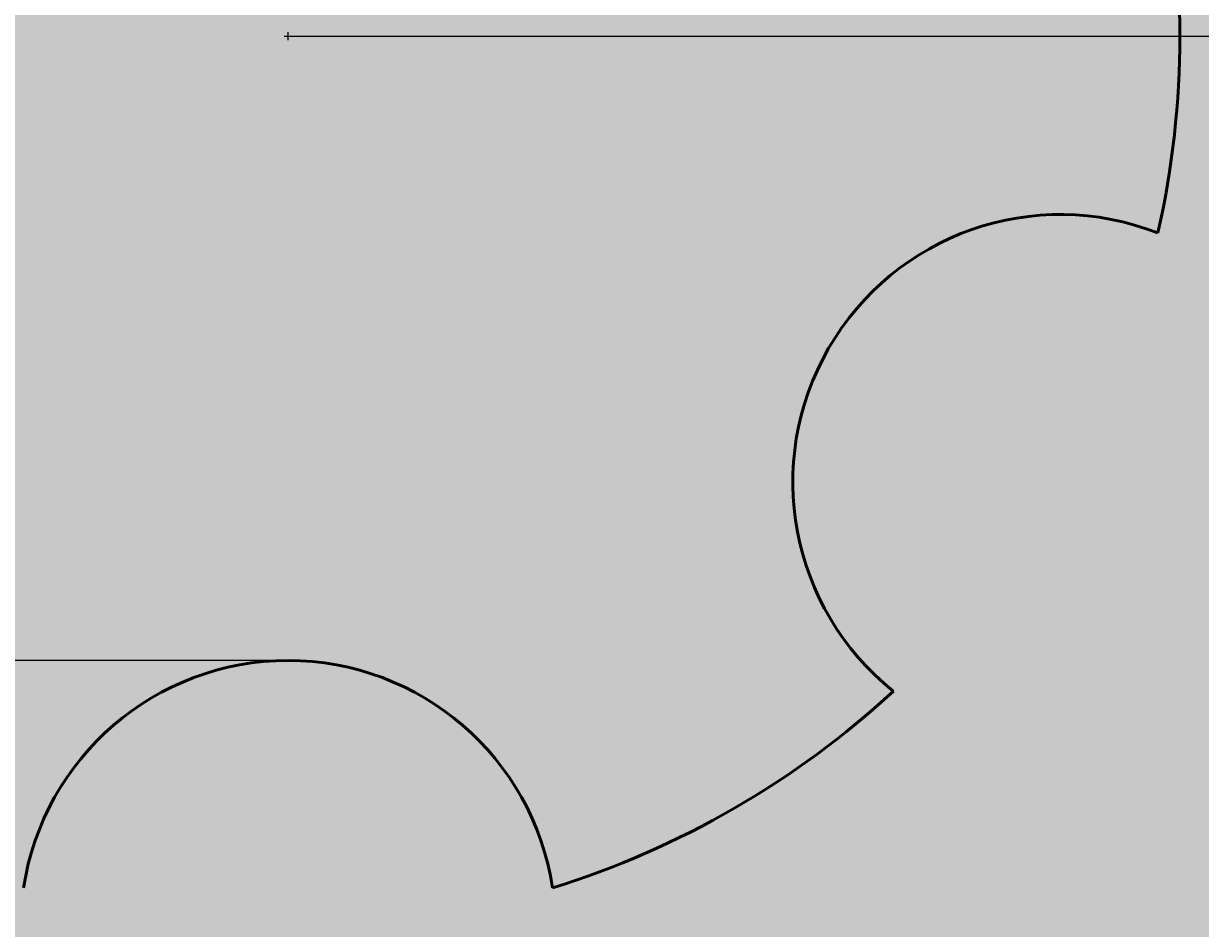
# Model space of a CAD drawing. Units: inches. Extents: x -13 to 107, y -48 to 102.
# Tile 6 of 13: x 22 to 48, y -7 to 14. Entities that reach past the tile are written whole.
import ezdxf

# ---------------------------------------------------------------- set-up
doc = ezdxf.new("R2010")
doc.units = ezdxf.units.IN
doc.header["$MEASUREMENT"] = 0
for name, color, linetype, lineweight in [('M-DIMS', 2, 'Continuous', 18), ('M-HATC', 8, 'Continuous', 18), ('M-OUTL', 7, 'Continuous', 50)]:
    doc.layers.add(name, color=color, linetype=linetype, lineweight=lineweight)
doc.styles.get("Standard").update_dxf_attribs({"font": 'arial.ttf'})
doc.dimstyles.get("Standard").update_dxf_attribs({"dimtxt": 0.18, "dimasz": 0.18, "dimexe": 0.18, "dimexo": 0.0625, "dimgap": 0.09, "dimtad": 0, "dimtih": 1, "dimtoh": 1, "dimdec": 4, "dimzin": 0, "dimdsep": 46, "dimtxsty": 'Standard', "dimcen": 0.09, "dimadec": 0, "dimazin": 0, "dimtfac": 1, "dimtdec": 4, "dimtofl": 0, "dimtmove": 0, "dimatfit": 3, "dimfxl": 1, "dimtolj": 1, "dimtzin": 0, "dimarcsym": 0})

# ---------------------------------------------------------------- blocks, each defined once
blk = doc.blocks.new('*D2')
at = {"layer": 'Defpoints', "color": 0, "transparency": 16777216}
for p in [(-12.585, 94.408), (27.547, 94.408), (27.547, -46.592)]:
    blk.add_point(p, dxfattribs=at)
at = {"layer": 'M-DIMS', "color": 0, "lineweight": -2, "transparency": 16777216}
for p, q in [((27.484, 94.408), (-12.765, 94.408)), ((-12.585, 94.228), (-12.585, 24.088)), ((-12.585, -46.412), (-12.585, 23.727)), ((27.484, -46.592), (-12.765, -46.592))]:
    blk.add_line(p, q, dxfattribs=at)
at = {"layer": 'M-DIMS', "color": 0, "transparency": 16777216}
for points in [[(-12.615, 94.228), (-12.555, 94.228), (-12.585, 94.408)], [(-12.615, -46.412), (-12.555, -46.412), (-12.585, -46.592)]]:
    blk.add_solid(points, dxfattribs=at)
at = {"layer": 'M-DIMS', "color": 0, "transparency": 16777216, "insert": (-12.585, 23.908), "char_height": 0.18, "attachment_point": 5}
blk.add_mtext('\\A1;141', dxfattribs=at)
blk = doc.blocks.new('*D3')
at = {"layer": 'Defpoints', "color": 0, "transparency": 16777216}
for p in [(27.547, 13.408), (67.679, 13.408), (27.547, -36.592)]:
    blk.add_point(p, dxfattribs=at)
at = {"layer": 'M-DIMS', "color": 0, "lineweight": -2, "transparency": 16777216}
for p, q in [((27.609, 13.408), (67.859, 13.408)), ((67.679, 13.228), (67.679, -11.41)), ((67.679, -36.412), (67.679, -11.774)), ((27.609, -36.592), (67.859, -36.592))]:
    blk.add_line(p, q, dxfattribs=at)
at = {"layer": 'M-DIMS', "color": 0, "transparency": 16777216}
for points in [[(67.649, 13.228), (67.709, 13.228), (67.679, 13.408)], [(67.649, -36.412), (67.709, -36.412), (67.679, -36.592)]]:
    blk.add_solid(points, dxfattribs=at)
at = {"layer": 'M-DIMS', "color": 0, "transparency": 16777216, "insert": (67.679, -11.592), "char_height": 0.18, "attachment_point": 5}
blk.add_mtext('\\A1;50', dxfattribs=at)
blk = doc.blocks.new('*D4')
at = {"layer": 'Defpoints', "color": 0, "transparency": 16777216}
for p in [(27.547, 78.408), (67.679, 78.408), (27.547, 13.408)]:
    blk.add_point(p, dxfattribs=at)
at = {"layer": 'M-DIMS', "color": 0, "lineweight": -2, "transparency": 16777216}
for p, q in [((27.609, 78.408), (67.859, 78.408)), ((67.679, 78.228), (67.679, 46.09)), ((67.679, 13.588), (67.679, 45.726)), ((27.609, 13.408), (67.859, 13.408))]:
    blk.add_line(p, q, dxfattribs=at)
at = {"layer": 'M-DIMS', "color": 0, "transparency": 16777216}
for points in [[(67.649, 78.228), (67.709, 78.228), (67.679, 78.408)], [(67.649, 13.588), (67.709, 13.588), (67.679, 13.408)]]:
    blk.add_solid(points, dxfattribs=at)
at = {"layer": 'M-DIMS', "color": 0, "transparency": 16777216, "insert": (67.679, 45.908), "char_height": 0.18, "attachment_point": 5}
blk.add_mtext('\\A1;65', dxfattribs=at)
blk = doc.blocks.new('*D5')
at = {"layer": 'Defpoints', "color": 0, "transparency": 16777216}
for p in [(20.412, 27.408), (27.547, 27.408), (27.547, -0.592)]:
    blk.add_point(p, dxfattribs=at)
at = {"layer": 'M-DIMS', "color": 0, "lineweight": -2, "transparency": 16777216}
for p, q in [((27.484, 27.408), (20.232, 27.408)), ((20.412, 27.228), (20.412, 13.59)), ((20.412, -0.412), (20.412, 13.226)), ((27.484, -0.592), (20.232, -0.592))]:
    blk.add_line(p, q, dxfattribs=at)
at = {"layer": 'M-DIMS', "color": 0, "transparency": 16777216}
for points in [[(20.382, 27.228), (20.442, 27.228), (20.412, 27.408)], [(20.382, -0.412), (20.442, -0.412), (20.412, -0.592)]]:
    blk.add_solid(points, dxfattribs=at)
at = {"layer": 'M-DIMS', "color": 0, "transparency": 16777216, "insert": (20.412, 13.408), "char_height": 0.18, "attachment_point": 5}
blk.add_mtext('\\A1;28', dxfattribs=at)
blk = doc.blocks.new('*D8')
at = {"layer": 'Defpoints', "color": 0, "transparency": 16777216}
for p in [(27.547, 13.408), (50.882, -9.927)]:
    blk.add_point(p, dxfattribs=at)
at = {"layer": 'M-DIMS', "color": 0, "lineweight": -2, "transparency": 16777216}
for p, q in [((27.547, 13.318), (27.547, 13.498)), ((27.457, 13.408), (27.637, 13.408)), ((64.882, -23.927), (51.009, -10.054)), ((65.062, -23.927), (64.882, -23.927))]:
    blk.add_line(p, q, dxfattribs=at)
at = {"layer": 'M-DIMS', "color": 0, "transparency": 16777216}
blk.add_solid([(51.03, -10.033), (50.988, -10.075), (50.882, -9.927)], dxfattribs=at)
at = {"layer": 'M-DIMS', "color": 0, "transparency": 16777216, "insert": (65.562, -23.927), "char_height": 0.18, "attachment_point": 5}
blk.add_mtext('\\A1;2X R33', dxfattribs=at)
blk = doc.blocks.new('*D9')
at = {"layer": 'Defpoints', "color": 0, "transparency": 16777216}
for p in [(17.547, 30.728), (27.547, 13.408)]:
    blk.add_point(p, dxfattribs=at)
at = {"layer": 'M-DIMS', "color": 0, "lineweight": -2, "transparency": 16777216}
for p, q in [((11.367, 41.121), (11.547, 41.121)), ((11.547, 41.121), (17.457, 30.884)), ((27.547, 13.318), (27.547, 13.498)), ((27.457, 13.408), (27.637, 13.408))]:
    blk.add_line(p, q, dxfattribs=at)
at = {"layer": 'M-DIMS', "color": 0, "transparency": 16777216}
blk.add_solid([(17.483, 30.899), (17.431, 30.869), (17.547, 30.728)], dxfattribs=at)
at = {"layer": 'M-DIMS', "color": 0, "transparency": 16777216, "insert": (10.868, 41.121), "char_height": 0.18, "attachment_point": 5}
blk.add_mtext('\\A1;6X R20', dxfattribs=at)

msp = doc.modelspace()

# ---------------------------------------------------------------- hatches: boundary and pattern name
at = {"layer": 'M-HATC'}
h = msp.add_hatch(color=256, dxfattribs=at)
h.set_gradient(color1=(88, 186, 72), color2=(241, 235, 31), tint=1)
h.paths.add_polyline_path([(45.86, -14.044, 0.420873), (54.577, 32.339, -0.184081), (43.437, 76.537, 1.124637), (11.657, 76.537, -0.184081), (0.517, 32.339, 0.420873), (9.234, -14.044, -0.304084), (17.743, -34.622, 1.220926), (37.351, -34.622, -0.304084)])
h.paths.add_polyline_path([(33.479, -5.692, 0.859727), (21.615, -5.692, -0.111692), (13.972, -1.28, 0.859727), (8.04, 8.995, -0.111692), (8.04, 17.82, 0.859727), (13.972, 28.095, -0.111692), (21.615, 32.508, 0.859727), (33.479, 32.508, -0.111692), (41.122, 28.095, 0.859727), (47.054, 17.82, -0.111692), (47.054, 8.995, 0.859727), (41.122, -1.28, -0.111692)], flags=16)
h.paths.add_polyline_path([(32.547, -36.592, -1), (22.547, -36.592, -1)], flags=16)
h.paths.add_polyline_path([(17.547, 78.408, -1), (37.547, 78.408, -1)], flags=16)
h = msp.add_hatch(color=256, dxfattribs=at)
h.set_gradient(color1=(0, 0, 255), tint=1)
h.paths.add_polyline_path([(47.054, 8.995, 0.111692), (47.054, 17.82, -0.859727), (41.122, 28.095, 0.111692), (33.479, 32.508, -0.859727), (21.615, 32.508, 0.111692), (13.972, 28.095, -0.859727), (8.04, 17.82, 0.111692), (8.04, 8.995, -0.859727), (13.972, -1.28, 0.111692), (21.615, -5.692, -0.859727), (33.479, -5.692, 0.111692), (41.122, -1.28, -0.859727)])
h.paths.add_polyline_path([(37.547, 78.408, 1), (17.547, 78.408, 1)])
h.paths.add_polyline_path([(32.547, -36.592, 1), (22.547, -36.592, 1)])

# ---------------------------------------------------------------- linework, layer by layer
at = {"layer": 'M-OUTL'}
for centre, radius, start, end in [((27.547, 13.408), 33, 303.707, 35.0067), ((27.547, 13.408), 20, 347.2539, 12.7461), ((44.867, 3.408), 6, 68.6269, 231.3731), ((27.547, -6.592), 6, 8.6269, 171.3731), ((27.547, 13.408), 20, 287.2539, 312.7461)]:
    msp.add_arc(centre, radius, start, end, dxfattribs=at)

# ---------------------------------------------------------------- dimensions: what is measured, and where the dimension line sits
at = {"layer": 'M-DIMS'}
for base, p1, p2, picture, middle in [((-12.585, 94.408), (27.547, -46.592), (27.547, 94.408), '*D2', (-12.585, 23.908)), ((67.679, 78.408), (27.547, 13.408), (27.547, 78.408), '*D4', (67.679, 45.908)), ((20.412, 27.408), (27.547, -0.592), (27.547, 27.408), '*D5', (20.412, 13.408)), ((67.679, 13.408), (27.547, -36.592), (27.547, 13.408), '*D3', (67.679, -11.592))]:
    dim = msp.add_linear_dim(base=base, p1=p1, p2=p2, angle=90, dimstyle='Standard', override={"dimdec": 0, "dimlfac": 1, "dimrnd": 0, "dimzin": 0, "dimdsep": 46, "dimlunit": 2}, dxfattribs=at)
    dim.commit()
    dim.dimension.update_dxf_attribs({"geometry": picture, "text_midpoint": middle})
for mpoint, text, picture, middle in [((17.547, 30.728), '6X <>', '*D9', (10.868, 41.121)), ((50.882, -9.927), '2X <>', '*D8', (65.562, -23.927))]:
    dim = msp.add_radius_dim(center=(27.547, 13.408), mpoint=mpoint, text=text, dimstyle='Standard', override={"dimdec": 0, "dimlfac": 1, "dimrnd": 0, "dimzin": 0, "dimdsep": 46, "dimlunit": 2}, dxfattribs=at)
    dim.commit()
    dim.dimension.update_dxf_attribs({"geometry": picture, "text_midpoint": middle, "dimtype": 164})

doc.saveas('drawing.dxf')
